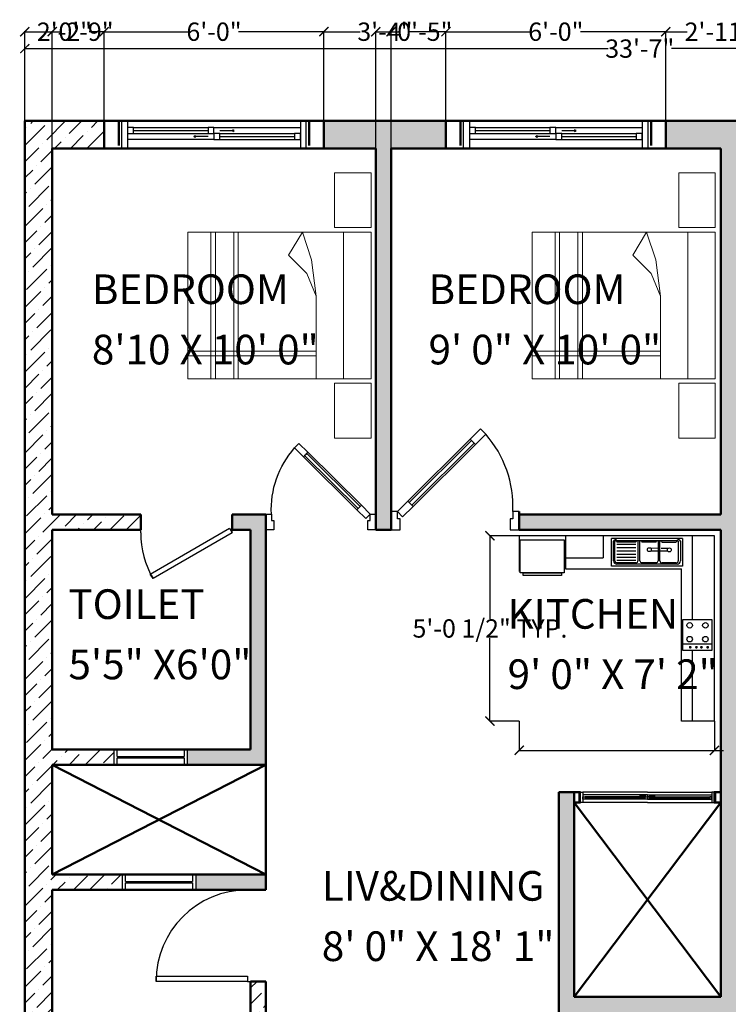
# Model space of a CAD drawing. Units: inches. Extents: x 2278 to 7495, y -71 to 1198.
# Tile 6 of 44: x 2844 to 3076, y 873 to 1195. Entities that reach past the tile are written whole.
import ezdxf

# ---------------------------------------------------------------- set-up
doc = ezdxf.new("R2010")
doc.units = ezdxf.units.IN
doc.header["$MEASUREMENT"] = 0
for name, color, linetype, lineweight in [('A-ANNO-DIMS', 2, 'Continuous', 18), ('A-AREA-IDEN', 3, 'Continuous', 18), ('A-Door', 3, 'Continuous', 25), ('A-FLOR-FIXT', 9, 'Continuous', 18), ('A-FURN', 8, 'Continuous', 18), ('A-Glaz', 4, 'Continuous', 25), ('A-Wall', 7, 'Continuous', 50), ('A-WALL-PATT', 8, 'Continuous', 18)]:
    doc.layers.add(name, color=color, linetype=linetype, lineweight=lineweight)
doc.layers.add('TEFRIŞ', color=11, linetype='Continuous')
doc.styles.get("Standard").update_dxf_attribs({"font": 'arial.ttf'})
doc.dimstyles.get("Standard").update_dxf_attribs({"dimtxt": 6, "dimasz": 3, "dimexe": 0.18, "dimexo": 0.0625, "dimgap": 0.09, "dimtad": 0, "dimtih": 1, "dimtoh": 1, "dimdec": 0, "dimzin": 0, "dimdsep": 46, "dimlunit": 3, "dimtxsty": 'Standard', "dimblk": 'ARCHTICK', "dimcen": 0.09, "dimadec": 0, "dimazin": 0, "dimtfac": 1, "dimtdec": 0, "dimtofl": 0, "dimtmove": 0, "dimatfit": 3, "dimfxl": 1, "dimtolj": 1, "dimtzin": 0, "dimarcsym": 0})

# ---------------------------------------------------------------- blocks, each defined once
blk = doc.blocks.new('A$C1DF4181C')
blk.add_lwpolyline([(120, 128), (460.7, 466.1), (432.5, 494.5), (91.8, 156.4)], close=True)
blk.add_arc((72.4, 128.7), 593.3, 357.2313, 41.4937)
at = {"layer": 'A-Door'}
for points in [[(517.5, 522.4), (460.7, 466.1), (432.5, 494.5), (489.3, 550.8)], [(63.2, 71.6), (120, 128), (91.8, 156.4), (35, 100)], [(35, 100), (0, 100), (0, 0), (50, 0), (50, 50), (50, 60), (35, 60)], [(665, 100), (665, 60), (650, 60), (650, 50), (650, 0), (700, 0), (700, 100)]]:
    blk.add_lwpolyline(points, close=True, dxfattribs=at)
at = {"layer": 'A-Glaz'}
blk.add_lwpolyline([(112.9, 135.1), (453.6, 473.2), (439.5, 487.4), (98.8, 149.3)], close=True, dxfattribs=at)
at = {"layer": 'A-Wall'}
for p, q in [((0, 0), (0, 100)), ((0, 100), (0, 0)), ((700, 0), (700, 100)), ((700, 0), (700, 100))]:
    blk.add_line(p, q, dxfattribs=at)
blk = doc.blocks.new('*U4')
for p, q in [((0, 0), (0, -6)), ((30, 0), (30, -6))]:
    blk.add_line(p, q)
blk.add_lwpolyline([(0, 0), (25.98, 15), (26.86, 13.48), (0.87, -1.52)], close=True)
blk.add_arc((0, 0), 30, 0, 30)
blk = doc.blocks.new('*U5')
for p, q in [((0, 0), (0, -6)), ((30, 0), (30, -6))]:
    blk.add_line(p, q)
blk.add_lwpolyline([(0, 0), (0, 30), (1.75, 30), (1.75, 0)], close=True)
blk.add_arc((0, 0), 30, 0, 90)
blk = doc.blocks.new('BED-160')
at = {"color": 0}
for p, q in [((-0.45, 2.35), (-0.45, 2.95)), ((-0.45, 2.95), (-0.05, 2.95)), ((-0.05, 2.95), (-0.05, 2.35)), ((-2.05, 2.3), (-0.05, 2.3)), ((-2.05, 0.7), (-2.05, 2.3)), ((-1.8, 0.7), (-1.8, 2.3)), ((-1.75, 0.7), (-1.75, 2.3)), ((-1.55, 0.7), (-1.55, 2.3)), ((-1.5, 0.7), (-1.5, 2.3)), ((-0.8, 2.3), (-0.95, 2.05)), ((-0.8, 2.3), (-0.7, 2)), ((-0.05, 2.35), (-0.45, 2.35)), ((-0.35, 0.7), (-0.35, 2.3)), ((-0.05, 2.3), (-0.05, 0.7)), ((-0.95, 2.05), (-0.75, 1.85)), ((-0.7, 2), (-0.65, 1.6)), ((-0.75, 1.85), (-0.65, 1.6)), ((-0.65, 1.6), (-0.65, 0.7)), ((-0.65, 1), (-2.05, 1)), ((-0.65, 0.95), (-2.05, 0.95)), ((-0.05, 0.7), (-2.05, 0.7)), ((-0.45, 0.65), (-0.05, 0.65)), ((-0.45, 0.05), (-0.45, 0.65)), ((-0.05, 0.65), (-0.05, 0.05)), ((-0.05, 0.05), (-0.45, 0.05))]:
    blk.add_line(p, q, dxfattribs=at)
blk = doc.blocks.new('A$C008029BD')
at = {"layer": 'TEFRIŞ', "ltscale": 0.05}
for p, q in [((0, 0), (0, -3.55)), ((3.37, 0), (0, 0)), ((3.37, 0), (3.37, -0.6)), ((1.522, -0.4), (0, -0.4)), ((3.37, -0.4), (2.083, -0.4)), ((0.05, -0.581), (0.05, -1.869)), ((0.05, -0.581), (0.55, -0.581)), ((0.086, -1.773), (0.086, -0.677)), ((0.096, -0.617), (0.454, -0.617)), ((0.099, -0.659), (0.457, -0.659)), ((0.113, -0.954), (0.113, -0.695)), ((0.493, -0.695), (0.493, -0.954)), ((0.514, -0.677), (0.514, -1.773)), ((0.55, -0.581), (0.55, -1.869)), ((0.6, -2.71), (0.6, -0.6)), ((3.37, -0.6), (0.6, -0.6)), ((0.23, -0.846), (0.229, -0.967)), ((0.28, -0.846), (0.277, -1.158)), ((0.096, -1.024), (0.454, -1.024)), ((0.457, -0.99), (0.099, -0.99)), ((0.11, -1.319), (0.11, -1.06)), ((0.228, -1.02), (0.227, -1.159)), ((0.49, -1.06), (0.49, -1.319)), ((0.454, -1.355), (0.096, -1.355)), ((0.096, -1.391), (0.454, -1.391)), ((0.11, -1.773), (0.11, -1.427)), ((0.154, -1.773), (0.154, -1.427)), ((0.214, -1.773), (0.214, -1.427)), ((0.274, -1.773), (0.274, -1.427)), ((0.334, -1.773), (0.334, -1.427)), ((0.39, -1.773), (0.39, -1.427)), ((0.444, -1.773), (0.444, -1.427)), ((0.49, -1.427), (0.49, -1.773)), ((0.55, -1.869), (0.05, -1.869)), ((0.454, -1.809), (0.096, -1.809)), ((0.454, -1.833), (0.096, -1.833)), ((0, -2.025), (0.4, -2.025)), ((0.4, -2.71), (0.4, -2.025)), ((0, -2.71), (0.6, -2.71)), ((0, -3.55), (0.65, -3.55))]:
    blk.add_line(p, q, dxfattribs=at)
at = {"layer": 'TEFRIŞ'}
blk.add_line((1.969, -0.05), (1.969, -0.572), dxfattribs=at)
at = {"layer": 'TEFRIŞ', "ltscale": 0.05}
for points in [[(1.522, -0.05), (2.083, -0.05), (2.083, -0.572), (1.522, -0.572)], [(0.67, -2.73), (0.67, -3.53), (0.07, -3.53), (0.07, -2.73)], [(0.72, -2.78), (0.72, -3.48), (0.67, -3.48), (0.67, -2.78)]]:
    blk.add_lwpolyline(points, close=True, dxfattribs=at)
at = {"layer": 'TEFRIŞ', "const_width": 0.025}
for points in [[(2.014, -0.123, 1), (2.039, -0.123, 1)], [(2.014, -0.236, 1), (2.039, -0.236, 1)], [(2.014, -0.327, 1), (2.039, -0.327, 1)], [(2.014, -0.44, 1), (2.039, -0.44, 1)]]:
    blk.add_lwpolyline(points, format="xyb", close=True, dxfattribs=at)
at = {"layer": 'TEFRIŞ', "ltscale": 0.05}
for centre, radius in [((1.628, -0.164), 0.0505), ((1.628, -0.45), 0.0505), ((0.255, -0.82), 0.036), ((0.252, -1.184), 0.036)]:
    blk.add_circle(centre, radius, dxfattribs=at)
at = {"layer": 'TEFRIŞ'}
for centre in [(1.88, -0.164), (1.88, -0.45)]:
    blk.add_circle(centre, 0.0505, dxfattribs=at)
at = {"layer": 'TEFRIŞ', "ltscale": 0.05}
for centre, radius, start, end in [((0.108, -0.649), 0.0351, 110.4976, 230.5777), ((0.118, -0.673), 0.023, 143.9853, 258.5157), ((0.454, -0.677), 0.06, 0, 90), ((0.457, -0.695), 0.036, 0, 90), ((0.115, -1.038), 0.023, 143.9853, 258.5157), ((0.118, -0.976), 0.023, 101.4843, 216.0147), ((0.454, -1.06), 0.036, 0, 90), ((0.457, -0.954), 0.036, 270, 0), ((0.115, -1.341), 0.023, 101.4843, 216.0147), ((0.115, -1.405), 0.023, 143.9853, 258.5157), ((0.454, -1.319), 0.036, 270, 0), ((0.454, -1.427), 0.036, 0, 90), ((0.108, -1.801), 0.0351, 129.4223, 249.5024), ((0.115, -1.796), 0.023, 101.4843, 216.0147), ((0.454, -1.773), 0.06, 270, 0), ((0.454, -1.773), 0.036, 270, 0)]:
    blk.add_arc(centre, radius, start, end, dxfattribs=at)
blk = doc.blocks.new('_ArchTick')
at = {"color": 0, "linetype": 'ByBlock', "const_width": 0.15}
blk.add_lwpolyline([(-0.5, -0.5), (0.5, 0.5)], dxfattribs=at)
blk = doc.blocks.new('*D36')
at = {"layer": 'A-ANNO-DIMS', "color": 0, "lineweight": -2, "transparency": 16777216}
for p, q in [((2845.93, 1162.32), (2845.93, 1186.15)), ((2845.93, 1185.97), (3037.04, 1185.97)), ((3248.93, 1185.97), (3057.82, 1185.97)), ((3248.93, 1162.32), (3248.93, 1186.15))]:
    blk.add_line(p, q, dxfattribs=at)
at = {"layer": 'Defpoints', "color": 0, "transparency": 16777216}
for p in [(3248.93, 1185.97), (2845.93, 1162.26), (3248.93, 1162.26)]:
    blk.add_point(p, dxfattribs=at)
at = {"layer": 'A-ANNO-DIMS', "color": 0, "lineweight": -2, "transparency": 16777216, "xscale": 3, "yscale": 3, "zscale": 3, "rotation": 180}
blk.add_blockref('_ArchTick', (2845.93, 1185.97), dxfattribs=at)
at = {"layer": 'A-ANNO-DIMS', "color": 0, "lineweight": -2, "transparency": 16777216, "xscale": 3, "yscale": 3, "zscale": 3}
blk.add_blockref('_ArchTick', (3248.93, 1185.97), dxfattribs=at)
at = {"layer": 'A-ANNO-DIMS', "color": 0, "transparency": 16777216, "insert": (3047.43, 1185.97), "char_height": 6, "attachment_point": 5}
blk.add_mtext('\\A1;33\'-7"', dxfattribs=at)
blk = doc.blocks.new('*D53')
at = {"layer": 'A-ANNO-DIMS', "color": 0, "lineweight": -2, "transparency": 16777216}
for p, q in [((3007.93, 965.51), (3007.93, 955.8)), ((3071.89, 965.51), (3071.89, 955.8)), ((3007.93, 955.98), (3071.89, 955.98)), ((3071.89, 955.98), (3074.89, 955.98))]:
    blk.add_line(p, q, dxfattribs=at)
at = {"layer": 'Defpoints', "color": 0, "transparency": 16777216}
for p in [(3007.93, 965.57), (3071.89, 965.57), (3071.89, 955.98)]:
    blk.add_point(p, dxfattribs=at)
at = {"layer": 'A-ANNO-DIMS', "color": 0, "lineweight": -2, "transparency": 16777216, "xscale": 3, "yscale": 3, "zscale": 3, "rotation": 180}
blk.add_blockref('_ArchTick', (3007.93, 955.98), dxfattribs=at)
at = {"layer": 'A-ANNO-DIMS', "color": 0, "lineweight": -2, "transparency": 16777216, "xscale": 3, "yscale": 3, "zscale": 3}
blk.add_blockref('_ArchTick', (3071.89, 955.98), dxfattribs=at)
at = {"layer": 'A-ANNO-DIMS', "color": 0, "transparency": 16777216, "insert": (3134.58, 955.98), "char_height": 6, "attachment_point": 5}
blk.add_mtext('\\A1;KITCHEN COUNTER 5\'-4" TYP.', dxfattribs=at)
blk = doc.blocks.new('*D54')
at = {"layer": 'A-ANNO-DIMS', "color": 0, "lineweight": -2, "transparency": 16777216}
for p, q in [((3007.87, 1026.29), (2998.16, 1026.29)), ((2998.34, 1026.29), (2998.34, 999.12)), ((2998.34, 965.57), (2998.34, 992.74)), ((3007.87, 965.57), (2998.16, 965.57))]:
    blk.add_line(p, q, dxfattribs=at)
at = {"layer": 'Defpoints', "color": 0, "transparency": 16777216}
for p in [(3007.93, 1026.29), (2998.34, 965.57), (3007.93, 965.57)]:
    blk.add_point(p, dxfattribs=at)
at = {"layer": 'A-ANNO-DIMS', "color": 0, "lineweight": -2, "transparency": 16777216, "xscale": 3, "yscale": 3, "zscale": 3}
for p, rotation in [((2998.34, 1026.29), 90), ((2998.34, 965.57), 270)]:
    blk.add_blockref('_ArchTick', p, dxfattribs=dict(at, rotation=rotation))
at = {"layer": 'A-ANNO-DIMS', "color": 0, "transparency": 16777216, "insert": (2998.34, 995.93), "char_height": 6, "attachment_point": 5}
blk.add_mtext('\\A1;5\'-0 1/2" TYP.', dxfattribs=at)
blk = doc.blocks.new('*D77')
at = {"layer": 'A-ANNO-DIMS', "color": 0, "lineweight": -2, "transparency": 16777216}
for p, q in [((2845.93, 1162.32), (2845.93, 1191.69)), ((2845.93, 1191.51), (2850.81, 1191.51)), ((2871.93, 1191.51), (2867.05, 1191.51)), ((2871.93, 1162.32), (2871.93, 1191.69))]:
    blk.add_line(p, q, dxfattribs=at)
at = {"layer": 'Defpoints', "color": 0, "transparency": 16777216}
for p in [(2871.93, 1191.51), (2845.93, 1162.26), (2871.93, 1162.26)]:
    blk.add_point(p, dxfattribs=at)
at = {"layer": 'A-ANNO-DIMS', "color": 0, "lineweight": -2, "transparency": 16777216, "xscale": 3, "yscale": 3, "zscale": 3, "rotation": 180}
blk.add_blockref('_ArchTick', (2845.93, 1191.51), dxfattribs=at)
at = {"layer": 'A-ANNO-DIMS', "color": 0, "lineweight": -2, "transparency": 16777216, "xscale": 3, "yscale": 3, "zscale": 3}
blk.add_blockref('_ArchTick', (2871.93, 1191.51), dxfattribs=at)
at = {"layer": 'A-ANNO-DIMS', "color": 0, "transparency": 16777216, "insert": (2858.93, 1191.51), "char_height": 6, "attachment_point": 5}
blk.add_mtext('\\A1;2\'-2"', dxfattribs=at)
blk = doc.blocks.new('*D78')
at = {"layer": 'A-ANNO-DIMS', "color": 0, "lineweight": -2, "transparency": 16777216}
for p, q in [((2871.93, 1162.32), (2871.93, 1191.69)), ((2871.93, 1191.51), (2899.85, 1191.51)), ((2943.93, 1191.51), (2916.01, 1191.51)), ((2943.93, 1162.32), (2943.93, 1191.69))]:
    blk.add_line(p, q, dxfattribs=at)
at = {"layer": 'Defpoints', "color": 0, "transparency": 16777216}
for p in [(2943.93, 1191.51), (2871.93, 1162.26), (2943.93, 1162.26)]:
    blk.add_point(p, dxfattribs=at)
at = {"layer": 'A-ANNO-DIMS', "color": 0, "lineweight": -2, "transparency": 16777216, "xscale": 3, "yscale": 3, "zscale": 3, "rotation": 180}
blk.add_blockref('_ArchTick', (2871.93, 1191.51), dxfattribs=at)
at = {"layer": 'A-ANNO-DIMS', "color": 0, "lineweight": -2, "transparency": 16777216, "xscale": 3, "yscale": 3, "zscale": 3}
blk.add_blockref('_ArchTick', (2943.93, 1191.51), dxfattribs=at)
at = {"layer": 'A-ANNO-DIMS', "color": 0, "transparency": 16777216, "insert": (2907.93, 1191.51), "char_height": 6, "attachment_point": 5}
blk.add_mtext('\\A1;6\'-0"', dxfattribs=at)
blk = doc.blocks.new('*D79')
at = {"layer": 'A-ANNO-DIMS', "color": 0, "lineweight": -2, "transparency": 16777216}
for p, q in [((2943.93, 1162.32), (2943.93, 1191.69)), ((2943.93, 1191.51), (2955.87, 1191.51)), ((2983.93, 1191.51), (2971.99, 1191.51)), ((2983.93, 1162.32), (2983.93, 1191.69))]:
    blk.add_line(p, q, dxfattribs=at)
at = {"layer": 'Defpoints', "color": 0, "transparency": 16777216}
for p in [(2983.93, 1191.51), (2943.93, 1162.26), (2983.93, 1162.26)]:
    blk.add_point(p, dxfattribs=at)
at = {"layer": 'A-ANNO-DIMS', "color": 0, "lineweight": -2, "transparency": 16777216, "xscale": 3, "yscale": 3, "zscale": 3, "rotation": 180}
blk.add_blockref('_ArchTick', (2943.93, 1191.51), dxfattribs=at)
at = {"layer": 'A-ANNO-DIMS', "color": 0, "lineweight": -2, "transparency": 16777216, "xscale": 3, "yscale": 3, "zscale": 3}
blk.add_blockref('_ArchTick', (2983.93, 1191.51), dxfattribs=at)
at = {"layer": 'A-ANNO-DIMS', "color": 0, "transparency": 16777216, "insert": (2963.93, 1191.51), "char_height": 6, "attachment_point": 5}
blk.add_mtext('\\A1;3\'-4"', dxfattribs=at)
blk = doc.blocks.new('*D80')
at = {"layer": 'A-ANNO-DIMS', "color": 0, "lineweight": -2, "transparency": 16777216}
for p, q in [((2983.93, 1162.32), (2983.93, 1191.69)), ((2983.93, 1191.51), (3011.85, 1191.51)), ((3055.93, 1191.51), (3028.01, 1191.51)), ((3055.93, 1162.32), (3055.93, 1191.69))]:
    blk.add_line(p, q, dxfattribs=at)
at = {"layer": 'Defpoints', "color": 0, "transparency": 16777216}
for p in [(3055.93, 1191.51), (2983.93, 1162.26), (3055.93, 1162.26)]:
    blk.add_point(p, dxfattribs=at)
at = {"layer": 'A-ANNO-DIMS', "color": 0, "lineweight": -2, "transparency": 16777216, "xscale": 3, "yscale": 3, "zscale": 3, "rotation": 180}
blk.add_blockref('_ArchTick', (2983.93, 1191.51), dxfattribs=at)
at = {"layer": 'A-ANNO-DIMS', "color": 0, "lineweight": -2, "transparency": 16777216, "xscale": 3, "yscale": 3, "zscale": 3}
blk.add_blockref('_ArchTick', (3055.93, 1191.51), dxfattribs=at)
at = {"layer": 'A-ANNO-DIMS', "color": 0, "transparency": 16777216, "insert": (3019.93, 1191.51), "char_height": 6, "attachment_point": 5}
blk.add_mtext('\\A1;6\'-0"', dxfattribs=at)
blk = doc.blocks.new('*D81')
at = {"layer": 'A-ANNO-DIMS', "color": 0, "lineweight": -2, "transparency": 16777216}
for p, q in [((3055.93, 1162.32), (3055.93, 1191.69)), ((3055.93, 1191.51), (3062.98, 1191.51)), ((3090.93, 1191.51), (3083.88, 1191.51)), ((3090.93, 1162.32), (3090.93, 1191.69))]:
    blk.add_line(p, q, dxfattribs=at)
at = {"layer": 'Defpoints', "color": 0, "transparency": 16777216}
for p in [(3090.93, 1191.51), (3055.93, 1162.26), (3090.93, 1162.26)]:
    blk.add_point(p, dxfattribs=at)
at = {"layer": 'A-ANNO-DIMS', "color": 0, "lineweight": -2, "transparency": 16777216, "xscale": 3, "yscale": 3, "zscale": 3, "rotation": 180}
blk.add_blockref('_ArchTick', (3055.93, 1191.51), dxfattribs=at)
at = {"layer": 'A-ANNO-DIMS', "color": 0, "lineweight": -2, "transparency": 16777216, "xscale": 3, "yscale": 3, "zscale": 3}
blk.add_blockref('_ArchTick', (3090.93, 1191.51), dxfattribs=at)
at = {"layer": 'A-ANNO-DIMS', "color": 0, "transparency": 16777216, "insert": (3073.43, 1191.51), "char_height": 6, "attachment_point": 5}
blk.add_mtext('\\A1;2\'-11"', dxfattribs=at)
blk = doc.blocks.new('*D91')
at = {"layer": 'A-ANNO-DIMS', "color": 0, "lineweight": -2, "transparency": 16777216}
for p, q in [((2845.93, 1162.32), (2845.93, 1191.69)), ((2845.93, 1191.51), (2854.93, 1191.51)), ((2854.93, 1153.32), (2854.93, 1191.69)), ((2854.93, 1191.51), (2857.93, 1191.51))]:
    blk.add_line(p, q, dxfattribs=at)
at = {"layer": 'Defpoints', "color": 0, "transparency": 16777216}
for p in [(2854.93, 1191.51), (2845.93, 1162.26), (2854.93, 1153.26)]:
    blk.add_point(p, dxfattribs=at)
at = {"layer": 'A-ANNO-DIMS', "color": 0, "lineweight": -2, "transparency": 16777216, "xscale": 3, "yscale": 3, "zscale": 3, "rotation": 180}
blk.add_blockref('_ArchTick', (2845.93, 1191.51), dxfattribs=at)
at = {"layer": 'A-ANNO-DIMS', "color": 0, "lineweight": -2, "transparency": 16777216, "xscale": 3, "yscale": 3, "zscale": 3}
blk.add_blockref('_ArchTick', (2854.93, 1191.51), dxfattribs=at)
at = {"layer": 'A-ANNO-DIMS', "color": 0, "transparency": 16777216, "insert": (2866, 1191.51), "char_height": 6, "attachment_point": 5}
blk.add_mtext('\\A1;0\'-9"', dxfattribs=at)
blk = doc.blocks.new('*D92')
at = {"layer": 'A-ANNO-DIMS', "color": 0, "lineweight": -2, "transparency": 16777216}
for p, q in [((2960.93, 1028.32), (2960.93, 1191.69)), ((2960.93, 1191.51), (2965.93, 1191.51)), ((2965.93, 1028.32), (2965.93, 1191.69)), ((2965.93, 1191.51), (2968.93, 1191.51))]:
    blk.add_line(p, q, dxfattribs=at)
at = {"layer": 'Defpoints', "color": 0, "transparency": 16777216}
for p in [(2965.93, 1191.51), (2960.93, 1028.26), (2965.93, 1028.26)]:
    blk.add_point(p, dxfattribs=at)
at = {"layer": 'A-ANNO-DIMS', "color": 0, "lineweight": -2, "transparency": 16777216, "xscale": 3, "yscale": 3, "zscale": 3, "rotation": 180}
blk.add_blockref('_ArchTick', (2960.93, 1191.51), dxfattribs=at)
at = {"layer": 'A-ANNO-DIMS', "color": 0, "lineweight": -2, "transparency": 16777216, "xscale": 3, "yscale": 3, "zscale": 3}
blk.add_blockref('_ArchTick', (2965.93, 1191.51), dxfattribs=at)
at = {"layer": 'A-ANNO-DIMS', "color": 0, "transparency": 16777216, "insert": (2977, 1191.51), "char_height": 6, "attachment_point": 5}
blk.add_mtext('\\A1;0\'-5"', dxfattribs=at)

msp = doc.modelspace()

# ---------------------------------------------------------------- hatches: boundary and pattern name
at = {"layer": 'A-WALL-PATT', "transparency": 33554687}
h = msp.add_hatch(dxfattribs=at)
h.set_pattern_fill('ANSI36', color=256, scale=30)
h.paths.add_polyline_path([(2854.93, 910.26), (2877.93, 910.26), (2877.93, 915.26), (2854.93, 915.26), (2854.93, 951.26), (2875.18, 951.26), (2875.18, 956.26), (2854.93, 956.26), (2854.93, 1028.26), (2883.93, 1028.26), (2883.93, 1033.26), (2854.93, 1033.26), (2854.93, 1153.26), (2871.93, 1153.26), (2871.93, 1162.26), (2845.93, 1162.26), (2845.93, 709.26), (2977.93, 709.26), (2977.93, 718.26), (2854.93, 718.26), (2854.93, 806.26), (2936.93, 806.26), (2936.93, 811.26), (2924.93, 811.26), (2924.93, 880.26), (2919.93, 880.26), (2919.93, 811.26), (2854.93, 811.26)])
h = msp.add_hatch(dxfattribs=at)
h.set_pattern_fill('ANSI36', color=256, scale=30)
h.paths.add_polyline_path([(3248.93, 883.76), (3239.93, 883.76), (3239.93, 881.26), (3119.93, 881.26), (3119.93, 916.26), (3114.93, 916.26), (3114.93, 876.26), (3239.93, 876.26), (3239.93, 759.26), (3195.43, 759.26), (3195.43, 754.26), (3248.93, 754.26)])
h.paths.add_polyline_path([(3248.93, 963.26), (3239.93, 963.26), (3114.93, 963.26), (3114.93, 952.26), (3119.93, 952.26), (3119.93, 958.26), (3239.93, 958.26), (3239.93, 955.76), (3248.93, 955.76)])
h.paths.add_polyline_path([(3078.93, 1076.26), (3090.93, 1076.26), (3090.93, 1081.26), (3078.93, 1081.26), (3078.93, 1153.26), (3090.93, 1153.26), (3090.93, 1162.26), (3055.93, 1162.26), (3055.93, 1153.26), (3073.93, 1153.26), (3073.93, 1033.26), (3007.93, 1033.26), (3007.93, 1028.26), (3073.93, 1028.26), (3073.93, 942.26), (3073.93, 938.92), (3073.93, 875.26), (3025.93, 875.26), (3025.93, 942.26), (3020.93, 942.26), (3020.93, 870.26), (3020.93, 864.53), (3025.94, 864.53), (3025.94, 870.26), (3073.93, 870.26), (3073.93, 804.26), (3078.93, 804.26)])
h.paths.add_polyline_path([(2983.93, 1162.26), (2943.93, 1162.26), (2943.93, 1153.26), (2960.93, 1153.26), (2960.93, 1033.26), (2960.93, 1028.26), (2965.93, 1028.26), (2965.93, 1153.26), (2983.93, 1153.26)])
h.paths.add_polyline_path([(3149.93, 1162.26), (3114.93, 1162.26), (3114.93, 1153.26), (3126.93, 1153.26), (3126.93, 1081.26), (3120.93, 1081.26), (3120.93, 1076.26), (3131.93, 1076.26), (3131.93, 1153.26), (3149.93, 1153.26)])
h.paths.add_polyline_path([(3248.93, 1162.26), (3221.93, 1162.26), (3221.93, 1153.26), (3239.93, 1153.26), (3239.93, 1040.26), (3126.93, 1040.26), (3126.93, 1035.26), (3239.93, 1035.26), (3248.93, 1035.26)])
h.paths.add_polyline_path([(3123.43, 759.26), (3078.93, 759.26), (3078.93, 762.26), (3073.93, 762.26), (3073.93, 754.26), (3123.43, 754.26)])
h.paths.add_polyline_path([(3025.93, 811.26), (3025.89, 817.61), (3020.93, 817.61), (3020.93, 811.26), (3008.93, 811.26), (3008.93, 806.26), (3025.93, 806.26)], flags=17)
h.paths.add_polyline_path([(2924.93, 1028.26), (2924.93, 1033.26), (2913.93, 1033.26), (2913.93, 1028.26), (2919.93, 1028.26), (2919.93, 956.26), (2899.18, 956.26), (2899.18, 951.26), (2924.93, 951.26)])
h.paths.add_polyline_path([(2924.93, 915.26), (2901.93, 915.26), (2901.93, 910.26), (2924.93, 910.26)])
h.paths.add_polyline_path([(3078.14, 1129.24), (3130.7, 1129.24), (3130.7, 1144.33), (3078.14, 1144.33)], flags=9)

# ---------------------------------------------------------------- linework, layer by layer
at = {"layer": 'A-Glaz'}
for p, q in [((2879.63, 1162.26), (2936.23, 1162.26)), ((2991.63, 1162.26), (3048.23, 1162.26)), ((2881.58, 1160.09), (2905.98, 1160.09)), ((2881.58, 1159.11), (2905.98, 1159.11)), ((2907.93, 1160.09), (2936.23, 1160.09)), ((2909.88, 1159.11), (2914.07, 1159.11)), ((2993.58, 1160.09), (3017.98, 1160.09)), ((2993.58, 1159.11), (3017.98, 1159.11)), ((3019.93, 1160.09), (3048.23, 1160.09)), ((3021.88, 1159.11), (3026.07, 1159.11)), ((2907.93, 1156.18), (2879.63, 1156.18)), ((2881.58, 1158.14), (2905.98, 1158.14)), ((2905.98, 1157.16), (2901.79, 1157.16)), ((2909.88, 1158.14), (2934.28, 1158.14)), ((2909.88, 1157.16), (2934.28, 1157.16)), ((2909.88, 1156.18), (2934.28, 1156.18)), ((3019.93, 1156.18), (2991.63, 1156.18)), ((2993.58, 1158.14), (3017.98, 1158.14)), ((3017.98, 1157.16), (3013.79, 1157.16)), ((3021.88, 1158.14), (3046.28, 1158.14)), ((3021.88, 1157.16), (3046.28, 1157.16)), ((3021.88, 1156.18), (3046.28, 1156.18)), ((2879.63, 1153.26), (2936.23, 1153.26)), ((2991.63, 1153.26), (3048.23, 1153.26)), ((2875.18, 956.26), (2899.18, 956.26)), ((2875.18, 951.26), (2875.18, 956.26)), ((2876.18, 953.96), (2876.18, 956.26)), ((2898.18, 956.26), (2898.18, 953.96)), ((2899.18, 956.26), (2899.18, 951.26)), ((2876.18, 953.96), (2898.18, 953.96)), ((2876.18, 951.26), (2876.18, 953.56)), ((2876.18, 953.56), (2898.18, 953.56)), ((2898.18, 953.56), (2898.18, 951.26)), ((2899.18, 951.26), (2875.18, 951.26)), ((3049.93, 942.26), (3028.78, 942.26)), ((3049.93, 942.26), (3071.08, 942.26)), ((3049.93, 941.45), (3028.78, 941.45)), ((3049.21, 940.73), (3029.51, 940.73)), ((3049.21, 940.37), (3029.51, 940.37)), ((3049.21, 940.01), (3029.51, 940.01)), ((3049.21, 941.09), (3047.66, 941.09)), ((3049.93, 941.45), (3071.08, 941.45)), ((3050.65, 941.09), (3052.21, 941.09)), ((3050.65, 940.73), (3070.36, 940.73)), ((3050.65, 940.37), (3070.36, 940.37)), ((3050.65, 940.01), (3070.36, 940.01)), ((3049.93, 938.92), (3028.78, 938.92)), ((3049.93, 938.92), (3071.08, 938.92)), ((2877.93, 915.26), (2901.93, 915.26)), ((2877.93, 910.26), (2877.93, 915.26)), ((2878.93, 912.96), (2878.93, 915.26)), ((2900.93, 915.26), (2900.93, 912.96)), ((2901.93, 915.26), (2901.93, 910.26)), ((2901.93, 910.26), (2877.93, 910.26)), ((2878.93, 912.96), (2900.93, 912.96)), ((2878.93, 910.26), (2878.93, 912.56)), ((2878.93, 912.56), (2900.93, 912.56)), ((2900.93, 912.56), (2900.93, 910.26))]:
    msp.add_line(p, q, dxfattribs=at)
for points in [[(2879.63, 1153.26), (2877.68, 1153.26), (2877.68, 1162.26), (2879.63, 1162.26)], [(2936.23, 1153.26), (2938.18, 1153.26), (2938.18, 1162.26), (2936.23, 1162.26)], [(2991.63, 1153.26), (2989.68, 1153.26), (2989.68, 1162.26), (2991.63, 1162.26)], [(3048.23, 1153.26), (3050.18, 1153.26), (3050.18, 1162.26), (3048.23, 1162.26)], [(2879.63, 1158.14), (2881.58, 1158.14), (2881.58, 1160.09), (2879.63, 1160.09)], [(2905.98, 1158.14), (2907.93, 1158.14), (2907.93, 1160.09), (2905.98, 1160.09)], [(2914.58, 1159.11), (2914.07, 1159.4), (2914.07, 1158.82)], [(2991.63, 1158.14), (2993.58, 1158.14), (2993.58, 1160.09), (2991.63, 1160.09)], [(3017.98, 1158.14), (3019.93, 1158.14), (3019.93, 1160.09), (3017.98, 1160.09)], [(3026.58, 1159.11), (3026.07, 1159.4), (3026.07, 1158.82)], [(2901.28, 1157.16), (2901.79, 1157.45), (2901.79, 1156.87)], [(2907.93, 1156.18), (2909.88, 1156.18), (2909.88, 1158.14), (2907.93, 1158.14)], [(2934.28, 1156.18), (2936.23, 1156.18), (2936.23, 1158.14), (2934.28, 1158.14)], [(3013.28, 1157.16), (3013.79, 1157.45), (3013.79, 1156.87)], [(3019.93, 1156.18), (3021.88, 1156.18), (3021.88, 1158.14), (3019.93, 1158.14)], [(3046.28, 1156.18), (3048.23, 1156.18), (3048.23, 1158.14), (3046.28, 1158.14)], [(3028.78, 938.92), (3028.06, 938.92), (3028.06, 942.26), (3028.78, 942.26)], [(3071.08, 938.92), (3071.8, 938.92), (3071.8, 942.26), (3071.08, 942.26)], [(3029.51, 940.01), (3028.78, 940.01), (3028.78, 940.73), (3029.51, 940.73)], [(3047.47, 941.09), (3047.66, 941.2), (3047.66, 940.98)], [(3049.21, 940.73), (3049.93, 940.73), (3049.93, 941.45), (3049.21, 941.45)], [(3049.93, 940.01), (3049.21, 940.01), (3049.21, 940.73), (3049.93, 940.73)], [(3050.65, 940.73), (3049.93, 940.73), (3049.93, 941.45), (3050.65, 941.45)], [(3049.93, 940.01), (3050.65, 940.01), (3050.65, 940.73), (3049.93, 940.73)], [(3052.39, 941.09), (3052.21, 941.2), (3052.21, 940.98)], [(3070.36, 940.01), (3071.08, 940.01), (3071.08, 940.73), (3070.36, 940.73)]]:
    msp.add_lwpolyline(points, close=True, dxfattribs=at)
at = {"layer": 'A-Wall'}
for p, q in [((2845.93, 1162.26), (2845.93, 709.26)), ((2845.93, 1162.26), (3248.93, 1162.26)), ((2871.93, 1153.26), (2871.93, 1162.26)), ((2877.68, 1162.26), (2871.93, 1162.26)), ((2876.7, 1162.04), (2876.7, 1154.23)), ((2938.18, 1162.26), (2943.93, 1162.26)), ((2939.16, 1162.04), (2939.16, 1154.23)), ((2943.93, 1153.26), (2943.93, 1162.26)), ((2983.93, 1153.26), (2983.93, 1162.26)), ((2989.68, 1162.26), (2983.93, 1162.26)), ((2988.7, 1162.04), (2988.7, 1154.23)), ((3050.18, 1162.26), (3055.93, 1162.26)), ((3051.16, 1162.04), (3051.16, 1154.23)), ((3055.93, 1153.26), (3055.93, 1162.26)), ((2854.93, 1153.26), (2854.93, 1033.26)), ((2854.93, 1153.26), (2960.93, 1153.26)), ((2877.68, 1153.26), (2871.93, 1153.26)), ((2938.18, 1153.26), (2943.93, 1153.26)), ((2960.93, 1153.26), (2960.93, 1033.26)), ((2965.93, 1153.26), (2965.93, 1028.26)), ((2965.93, 1153.26), (3073.93, 1153.26)), ((2989.68, 1153.26), (2983.93, 1153.26)), ((3050.18, 1153.26), (3055.93, 1153.26)), ((3073.93, 1153.26), (3073.93, 1033.26)), ((2854.93, 1033.26), (2883.93, 1033.26)), ((2883.93, 1028.26), (2883.93, 1033.26)), ((2913.93, 1033.26), (2924.93, 1033.26)), ((2913.93, 1028.26), (2913.93, 1033.26)), ((2924.93, 1033.26), (2924.93, 1028.26)), ((2960.93, 1033.26), (2960.93, 1028.26)), ((3007.93, 1033.26), (3073.93, 1033.26)), ((3007.93, 1028.26), (3007.93, 1033.26)), ((2854.93, 1028.26), (2854.93, 956.26)), ((2854.93, 1028.26), (2883.93, 1028.26)), ((2913.93, 1028.26), (2919.93, 1028.26)), ((2919.93, 1028.26), (2919.93, 956.26)), ((2924.93, 1028.26), (2924.93, 910.26)), ((2960.93, 1028.26), (2965.93, 1028.26)), ((3007.93, 1028.26), (3073.93, 1028.26)), ((3073.93, 1028.26), (3073.93, 942.26)), ((2854.93, 956.26), (2919.93, 956.26)), ((2854.93, 951.26), (2854.93, 915.26)), ((2854.93, 951.26), (2924.93, 951.26)), ((2924.93, 915.26), (2854.93, 951.26)), ((2854.93, 915.26), (2924.93, 951.26)), ((3020.93, 942.26), (3020.93, 870.26)), ((3025.93, 942.26), (3020.93, 942.26)), ((3025.93, 942.26), (3025.93, 875.26)), ((3025.93, 938.92), (3025.93, 942.26)), ((3028.06, 942.26), (3025.93, 942.26)), ((3071.8, 942.26), (3073.93, 942.26)), ((3073.93, 942.26), (3073.93, 875.26)), ((3073.93, 938.92), (3073.93, 942.26)), ((3027.7, 942.18), (3027.7, 939.29)), ((3072.16, 942.18), (3072.16, 939.29)), ((3028.06, 938.92), (3025.93, 938.92)), ((3025.93, 875.26), (3073.93, 938.92)), ((3073.93, 875.26), (3025.93, 938.92)), ((3071.8, 938.92), (3073.93, 938.92)), ((2854.93, 915.26), (2924.93, 915.26)), ((2854.93, 910.26), (2854.93, 811.26)), ((2854.93, 910.26), (2924.93, 910.26)), ((2919.93, 880.26), (2919.93, 811.26)), ((2919.93, 880.26), (2924.93, 880.26)), ((2924.93, 880.26), (2924.93, 811.26)), ((3025.93, 875.26), (3073.93, 875.26))]:
    msp.add_line(p, q, dxfattribs=at)

# ---------------------------------------------------------------- block references
at = {"layer": 'A-Door'}
for p, xscale, yscale, zscale in [((2965.93, 1028.26), 0.0599999999999766, 0.0599999999999766, 0.0599999999999766), ((2960.93, 1028.26), -0.051428571401403, 0.051428571401403, 0.051428571401403)]:
    msp.add_blockref('A$C1DF4181C', p, dxfattribs=dict(at, xscale=xscale, yscale=yscale, zscale=zscale))
for name, p, rotation in [('*U4', (2913.93, 1027.26), 180), ('*U5', (2918.93, 880.26), 89.99999999999999)]:
    msp.add_blockref(name, p, dxfattribs=dict(at, rotation=rotation))
at = {"layer": 'A-FLOR-FIXT', "xscale": 18.01737512370223, "yscale": 18.01737512370223, "zscale": 18.01737512370223, "rotation": 270}
msp.add_blockref('A$C008029BD', (3071.89, 1026.29), dxfattribs=at)
at = {"layer": 'A-FURN', "xscale": 29.9999999999997, "yscale": 29.9999999999997, "zscale": 29.9999999999997}
for p in [(2960.88, 1056.79), (3073.67, 1056.79)]:
    msp.add_blockref('BED-160', p, dxfattribs=at)

# ---------------------------------------------------------------- texts
at = {"layer": 'A-AREA-IDEN'}
for s, height, p in [('BEDROOM', 9.72, (2867.92, 1102.24)), ('BEDROOM', 9.72, (2978.22, 1102.24)), ('8\'10 X 10\' 0"', 9.7203, (2867.92, 1082.47)), ('9\' 0" X 10\' 0"', 9.7203, (2978.22, 1082.47)), ('TOILET', 9.72, (2860.24, 999.04)), ('KITCHEN', 9.72, (3004.12, 995.85)), ('5\'5" X6\'0"', 9.72, (2860.24, 979.27)), ('9\' 0" X 7\' 2"', 9.7203, (3004.12, 976.08)), ('LIV&DINING', 9.72, (2943.25, 906.71)), ('8\' 0" X 18\' 1"', 9.7203, (2943.25, 886.94))]:
    msp.add_text(s, height=height, dxfattribs=at).set_placement(p)

# ---------------------------------------------------------------- dimensions: what is measured, and where the dimension line sits
at = {"layer": 'A-ANNO-DIMS'}
for base, p1, p2, override, picture, middle in [((2871.93, 1191.51), (2845.93, 1162.26), (2871.93, 1162.26), {"dimdec": 1, "dimlfac": 1, "dimrnd": 0, "dimzin": 1, "dimdsep": 46, "dimlunit": 4, "dimfrac": 2}, '*D77', (2858.93, 1191.51)), ((2854.93, 1191.51), (2845.93, 1162.26), (2854.93, 1153.26), {"dimdec": 1, "dimlfac": 1, "dimrnd": 0, "dimzin": 1, "dimdsep": 46, "dimlunit": 4, "dimfrac": 2}, '*D91', (2866, 1191.51)), ((2943.93, 1191.51), (2871.93, 1162.26), (2943.93, 1162.26), {"dimdec": 1, "dimlfac": 1, "dimrnd": 0, "dimzin": 1, "dimdsep": 46, "dimlunit": 4, "dimfrac": 2}, '*D78', (2907.93, 1191.51)), ((2983.93, 1191.51), (2943.93, 1162.26), (2983.93, 1162.26), {"dimdec": 1, "dimlfac": 1, "dimrnd": 0, "dimzin": 1, "dimdsep": 46, "dimlunit": 4, "dimfrac": 2}, '*D79', (2963.93, 1191.51)), ((2965.93, 1191.51), (2960.93, 1028.26), (2965.93, 1028.26), {"dimdec": 1, "dimlfac": 1, "dimrnd": 0, "dimzin": 1, "dimdsep": 46, "dimlunit": 4, "dimfrac": 2}, '*D92', (2977, 1191.51)), ((3055.93, 1191.51), (2983.93, 1162.26), (3055.93, 1162.26), {"dimdec": 1, "dimlfac": 1, "dimrnd": 0, "dimzin": 1, "dimdsep": 46, "dimlunit": 4, "dimfrac": 2}, '*D80', (3019.93, 1191.51)), ((3090.93, 1191.51), (3055.93, 1162.26), (3090.93, 1162.26), {"dimdec": 1, "dimlfac": 1, "dimrnd": 0, "dimzin": 1, "dimdsep": 46, "dimlunit": 4, "dimfrac": 2}, '*D81', (3073.43, 1191.51)), ((3248.93, 1185.97), (2845.93, 1162.26), (3248.93, 1162.26), {"dimclrd": 0, "dimclre": 0, "dimclrt": 0}, '*D36', (3047.43, 1185.97))]:
    dim = msp.add_linear_dim(base=base, p1=p1, p2=p2, dimstyle='Standard', override=override, dxfattribs=at)
    dim.commit()
    dim.dimension.update_dxf_attribs({"geometry": picture, "text_midpoint": middle})
dim = msp.add_linear_dim(base=(2998.34, 965.57), p1=(3007.93, 1026.29), p2=(3007.93, 965.57), angle=270, text='<> TYP.', dimstyle='Standard', override={"dimdec": 1, "dimrnd": 0, "dimzin": 1, "dimlunit": 4, "dimfrac": 2}, dxfattribs=at)
dim.commit()
dim.dimension.update_dxf_attribs({"geometry": '*D54', "text_midpoint": (2998.34, 995.93)})
dim = msp.add_linear_dim(base=(3071.89, 955.98), p1=(3007.93, 965.57), p2=(3071.89, 965.57), text='KITCHEN COUNTER <> TYP.', dimstyle='Standard', override={"dimdec": 1, "dimrnd": 0, "dimzin": 1, "dimlunit": 4, "dimfrac": 2}, dxfattribs=at)
dim.commit()
dim.dimension.update_dxf_attribs({"geometry": '*D53', "text_midpoint": (3134.58, 955.98)})

doc.saveas('drawing.dxf')
